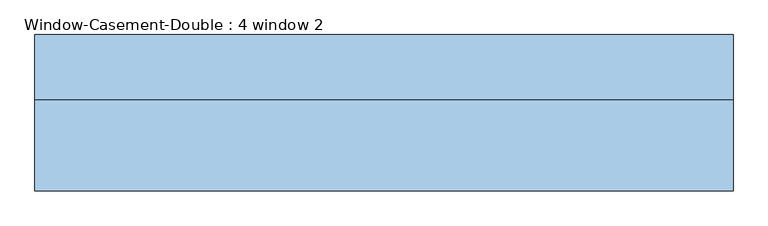
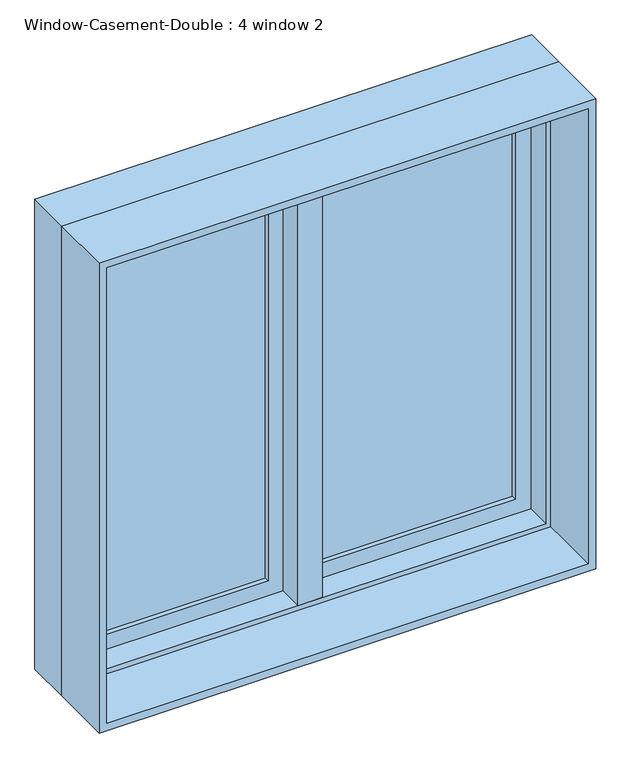
"""IFC4 building model written with IfcOpenShell, lengths in millimetres: window geometry, Window-Casement-Double : 4 window 2."""

from ifc_helpers import new_model, si_unit, frame, origin, place, context, project, spatial, polyline, outline, extrude, faceted_brep, source, transform, mapped, element, save


def window_casement_double_4_window_2_5590f608(model_context):
    return source(origin(), model_context, "Body", "SolidModel", [
        faceted_brep([(9.525, 146.05, 2120.9), (-9.525, 146.05, 2120.9), (-9.525, 95.25, 2120.9), (9.525, 95.25, 2120.9), (9.525, 146.05, 927.1), (9.525, 95.25, 927.1), (-9.525, 95.25, 927.1), (-9.525, 146.05, 927.1), (-9.525, 95.25, 946.15), (-9.525, 95.25, 2101.85), (-30.1625, 95.25, 946.15), (-30.1625, 95.25, 2101.85), (-30.1625, 31.75, 946.15), (-30.1625, 31.75, 2101.85), (30.1625, 31.75, 946.15), (30.1625, 31.75, 2101.85), (30.1625, 95.25, 946.15), (30.1625, 95.25, 2101.85), (9.525, 95.25, 946.15), (9.525, 95.25, 2101.85)], [[[0, 1, 2, 3]], [[4, 5, 6, 7]], [[1, 0, 4, 7]], [[2, 1, 7, 6, 8, 9]], [[9, 8, 10, 11]], [[11, 10, 12, 13]], [[13, 12, 14, 15]], [[15, 14, 16, 17]], [[17, 16, 18, 19]], [[0, 3, 19, 18, 5, 4]], [[18, 8, 6, 5]], [[9, 19, 3, 2]], [[8, 18, 16, 14, 12, 10]], [[19, 9, 11, 13, 15, 17]]]),
        extrude(outline(polyline([(-66.675, 127.0), (-66.675, 120.65), (-539.75, 120.65), (-539.75, 127.0), (-66.675, 127.0)])), frame((0.0, 0.0, 984.25), z_axis=(0.0, 0.0, 1.0), x_axis=(1.0, 0.0, 0.0)), (0.0, 0.0, 1.0), 1079.5),
        extrude(outline(polyline([(-539.75, 107.95), (-539.75, 114.3), (-66.675, 114.3), (-66.675, 107.95), (-539.75, 107.95)])), frame((0.0, 0.0, 984.25), z_axis=(0.0, 0.0, 1.0), x_axis=(1.0, 0.0, 0.0)), (0.0, 0.0, 1.0), 1079.5),
        extrude(outline(polyline([(539.75, 127.0), (539.75, 120.65), (66.675, 120.65), (66.675, 127.0), (539.75, 127.0)])), frame((0.0, 0.0, 984.25), z_axis=(0.0, 0.0, 1.0), x_axis=(1.0, 0.0, 0.0)), (0.0, 0.0, 1.0), 1079.5),
        extrude(outline(polyline([(66.675, 107.95), (66.675, 114.3), (539.75, 114.3), (539.75, 107.95), (66.675, 107.95)])), frame((0.0, 0.0, 984.25), z_axis=(0.0, 0.0, 1.0), x_axis=(1.0, 0.0, 0.0)), (0.0, 0.0, 1.0), 1079.5),
        extrude(outline(polyline([(2120.9, -596.9), (927.1, -596.9), (927.1, -9.525), (2120.9, -9.525), (2120.9, -596.9)]), holes=[polyline([(2063.75, -66.675), (984.25, -66.675), (984.25, -539.75), (2063.75, -539.75), (2063.75, -66.675)])]), frame((0.0, 95.25, 0.0), z_axis=(0.0, 1.0, 0.0), x_axis=(0.0, 0.0, 1.0)), (0.0, 0.0, 1.0), 44.45),
        extrude(outline(polyline([(927.1, 596.9), (2120.9, 596.9), (2120.9, 9.525), (927.1, 9.525), (927.1, 596.9)]), holes=[polyline([(984.25, 66.675), (2063.75, 66.675), (2063.75, 539.75), (984.25, 539.75), (984.25, 66.675)])]), frame((0.0, 95.25, 0.0), z_axis=(0.0, 1.0, 0.0), x_axis=(0.0, 0.0, 1.0)), (0.0, 0.0, 1.0), 44.45),
        extrude(outline(polyline([(2133.6, -609.6), (914.4, -609.6), (914.4, 609.6), (2133.6, 609.6), (2133.6, -609.6)]), holes=[polyline([(2114.55, 590.55), (933.45, 590.55), (933.45, -590.55), (2114.55, -590.55), (2114.55, 590.55)])]), frame((0.0, -127.0, 0.0), z_axis=(0.0, 1.0, 0.0), x_axis=(0.0, 0.0, 1.0)), (0.0, 0.0, 1.0), 158.75),
        faceted_brep([(577.85, 95.25, 2101.85), (577.85, 31.75, 2101.85), (-577.85, 31.75, 2101.85), (-577.85, 95.25, 2101.85), (596.9, 146.05, 2120.9), (596.9, 95.25, 2120.9), (-596.9, 95.25, 2120.9), (-596.9, 146.05, 2120.9), (609.6, 31.75, 2133.6), (609.6, 146.05, 2133.6), (-609.6, 146.05, 2133.6), (-609.6, 31.75, 2133.6), (-577.85, 31.75, 946.15), (-577.85, 95.25, 946.15), (-596.9, 95.25, 927.1), (-596.9, 146.05, 927.1), (-609.6, 146.05, 914.4), (-609.6, 31.75, 914.4), (577.85, 31.75, 946.15), (577.85, 95.25, 946.15), (596.9, 95.25, 927.1), (596.9, 146.05, 927.1), (609.6, 146.05, 914.4), (609.6, 31.75, 914.4)], [[[0, 1, 2, 3]], [[4, 5, 6, 7]], [[8, 9, 10, 11]], [[3, 2, 12, 13]], [[7, 6, 14, 15]], [[11, 10, 16, 17]], [[13, 12, 18, 19]], [[15, 14, 20, 21]], [[17, 16, 22, 23]], [[11, 17, 23, 8], [1, 18, 12, 2]], [[19, 18, 1, 0]], [[5, 20, 14, 6], [3, 13, 19, 0]], [[21, 20, 5, 4]], [[23, 22, 9, 8]], [[9, 22, 16, 10], [7, 15, 21, 4]]]),
    ])


if __name__ == "__main__":
    model = new_model("IFC4")
    model_context = context("Model", 3, world=origin())
    ifc_project = project(units=[si_unit("LENGTHUNIT", "METRE", prefix="MILLI")], contexts=[model_context])
    site = spatial("IfcSite", under=ifc_project)
    building = spatial("IfcBuilding", under=site)
    placement = place(None, origin())
    window_casement_double_4_window_2_shape = window_casement_double_4_window_2_5590f608(model_context)
    element("IfcWindow", 1, ObjectType="Window-Casement-Double : 4 window 2", at=placement, inside=building, context=model_context, shape_type="MappedRepresentation", body=[
        mapped(window_casement_double_4_window_2_shape, transform((0.0, 0.0, 0.0), x_axis=(1.0, 0.0, 0.0), y_axis=(0.0, 1.0, 0.0), z_axis=(0.0, 0.0, 1.0))),
    ])
    save(model, "model.ifc")

# Revit data of these elements
# Type "Window-Casement-Double : 4 window 2"
#   Type Mark = "22"
#   Fire Rating = "0.5h"
#   Assembly Code = "B2020100"
#   Analytic Construction = "Double glazing - domestic"
#   Frame Extension [instance default] = 0' - 0 1/4"
#   Window Inset [instance default] = 0' - 0"
#   Wall Thickness [instance default] = 0' - 6"
#   Interior Wall Closure [instance default] = 0' - 2 1/4"
#   Half Width = 2' - 0"
#   Visual Light Transmittance = 0.81
#   Thermal Resistance (R) = 1.8146 (h·ft²·°F)/BTU
#   Solar Heat Gain Coefficient = 0.76
#   Rough Width = 4' - 0 1/2"
#   Rough Height = 4' - 0 1/2"
#   Height = 4' - 0"
#   Heat Transfer Coefficient (U) = 0.5511 BTU/(h·ft²·°F)
#   Exterior Wall Closure [instance default] = 0' - 1 1/4"
#   Extension Jamb [instance default] = 0' - 2 1/4"
#   Default Sill Height = 3' - 0"
#   Width = 4' - 0"
#   Muntin Visibility = yes
#   Interior Trim Visibility [instance default] = yes
#   Exterior Trim Visibility [instance default] = yes
#   Extension Jamb Visibility [instance default] = yes
#   Interior Trim Material = Wood - Stained
#   Muntin Pattern = Muntin Pattern_2x2 : Muntin Pattern_2x2
#   Interior Trim = Trim-Window-Interior-Flat : Picture Frame
#   Interior Frame Material = Wood - Stained
#   Glass Panel Material = Glass
#   Exterior Trim Material = Clad - White
#   Exterior Trim = Trim-Window-Exterior-Flat : with Sill
#   Exterior Frame Material = Clad - White
#   Wall Closure = (empty or 0)
# Element 1 (IfcWindow, "Window-Casement-Double : 4 window 2")
#   Wall Thickness = 0' - 10"
#   Extension Jamb = 0' - 6 1/4"
#   Materials on its faces: "Wood - Stained", "Glass", "Clad - White"
# Materials
#   "Wood - Stained": class "Wood", colour RGB 224 178 126, transparency 0, Cost = 0
#   "Glass": class "Glass", colour RGB 0 128 192, transparency 0.75, Description = "Soda Lime Glass", Cost = 0
#   "Clad - White": class "Wood", colour RGB 242 242 238, transparency 0, Cost = 0
